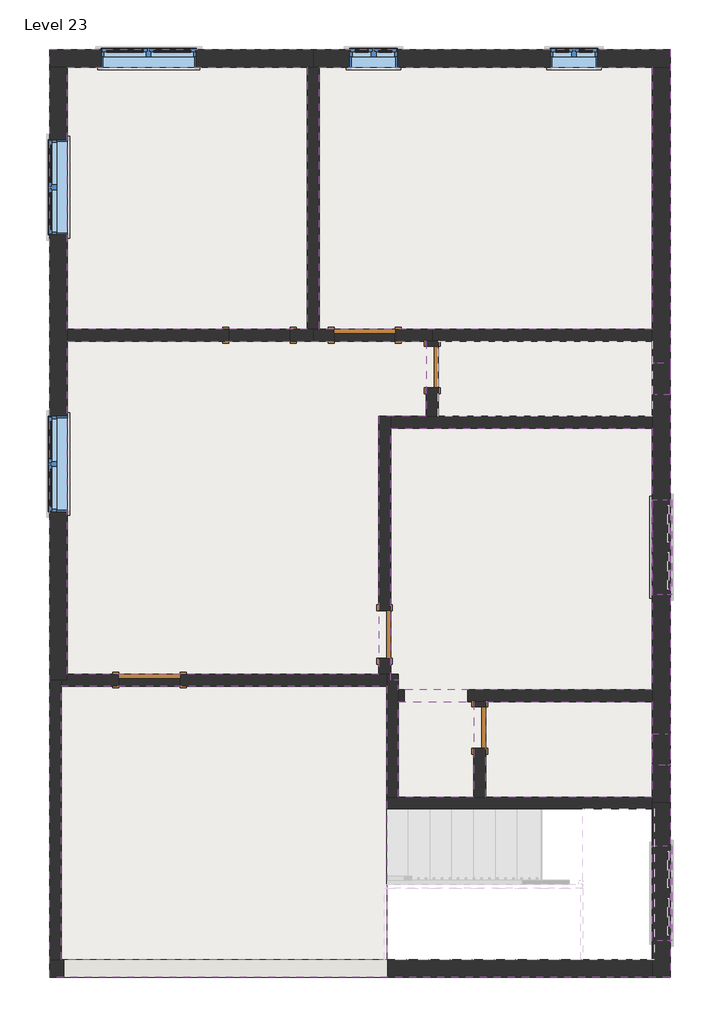
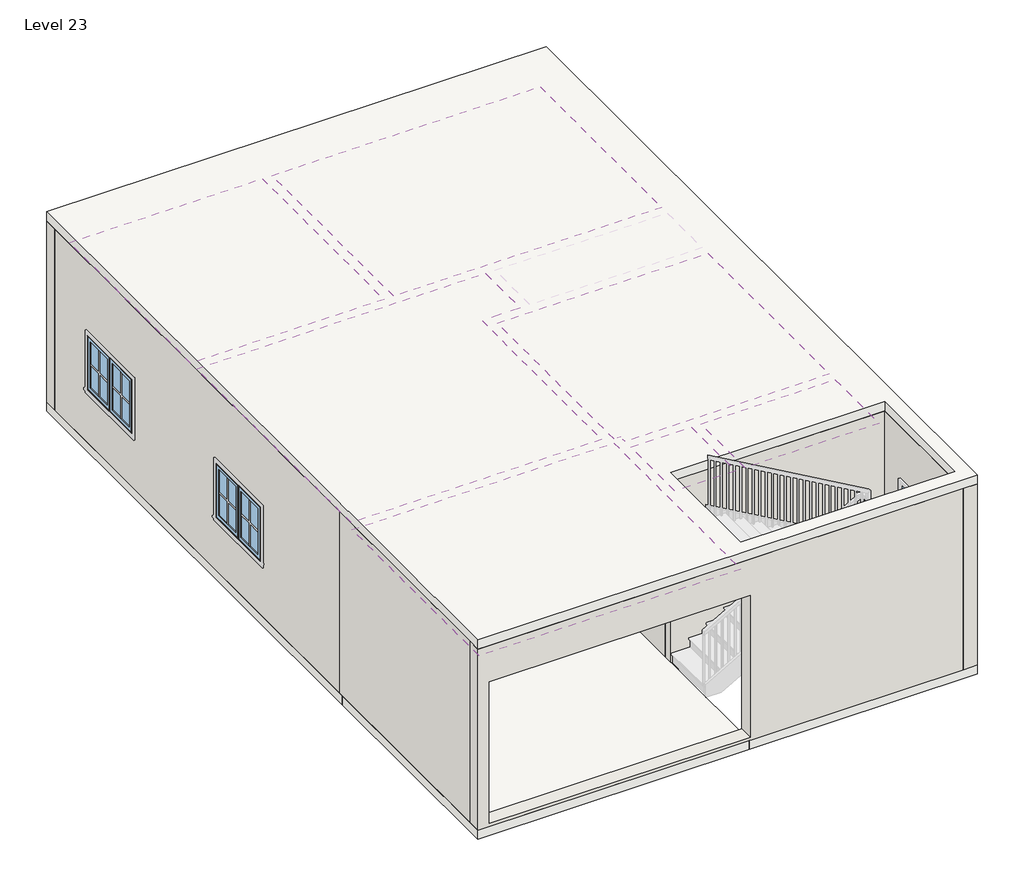
# One storey, part 1 of 2: 27 walls, 13 windows, 7 coverings, 6 doors, 3 slabs.
# Revit data of these elements (continued)
# Element 47 (IfcWindow, "Window-Casement-Double : 3'") (continued)
#   Materials on its faces: "Wood - Stained", "Glass", "Clad - White"
# Element 48 (IfcWindow, "Window-Casement-Double : 3'")
#   Mark = "103"
#   Window Inset = 0' - 0"
#   Interior Wall Closure = 0' - 2 1/4"
#   Frame Extension = 0' - 0 1/4"
#   Exterior Wall Closure = 0' - 1 1/4"
#   Interior Trim Visibility = yes
#   Exterior Trim Visibility = yes
#   Phase Created = New Construction
#   Materials on its faces: "Wood - Stained", "Glass", "Clad - White"
# Element 49 (IfcWindow, "Window-Casement-Double : 3'")
#   Mark = "104"
#   Window Inset = 0' - 0"
#   Interior Wall Closure = 0' - 2 1/4"
#   Frame Extension = 0' - 0 1/4"
#   Exterior Wall Closure = 0' - 1 1/4"
#   Interior Trim Visibility = yes
#   Exterior Trim Visibility = yes
#   Phase Created = New Construction
#   Materials on its faces: "Wood - Stained", "Glass", "Clad - White"
# Element 50 (IfcWindow, "Window-Casement-Double : 4'")
#   Mark = "92"
#   Window Inset = 0' - 0"
#   Interior Wall Closure = 0' - 2 1/4"
#   Frame Extension = 0' - 0 1/4"
#   Exterior Wall Closure = 0' - 1 1/4"
#   Interior Trim Visibility = yes
#   Exterior Trim Visibility = yes
#   Phase Created = New Construction
#   Materials on its faces: "Wood - Stained", "Glass", "Clad - White"
# Element 51 (IfcWindow, "Window-Casement-Double : 4'")
#   Mark = "93"
#   Window Inset = 0' - 0"
#   Interior Wall Closure = 0' - 2 1/4"
#   Frame Extension = 0' - 0 1/4"
#   Exterior Wall Closure = 0' - 1 1/4"
#   Interior Trim Visibility = yes
#   Exterior Trim Visibility = yes
#   Phase Created = New Construction
#   Materials on its faces: "Wood - Stained", "Glass", "Clad - White"
# Element 52 (IfcWindow, "Window-Casement-Double : 4'")
#   Mark = "94"
#   Window Inset = 0' - 0"
#   Interior Wall Closure = 0' - 2 1/4"
#   Frame Extension = 0' - 0 1/4"
#   Exterior Wall Closure = 0' - 1 1/4"
#   Interior Trim Visibility = yes
#   Exterior Trim Visibility = yes
#   Phase Created = New Construction
#   Materials on its faces: "Wood - Stained", "Glass", "Clad - White"
# Element 53 (IfcWindow, "Window-Casement-Double : 4'")
#   Mark = "95"
#   Window Inset = 0' - 0"
#   Interior Wall Closure = 0' - 2 1/4"
#   Frame Extension = 0' - 0 1/4"
#   Exterior Wall Closure = 0' - 1 1/4"
#   Interior Trim Visibility = yes
#   Exterior Trim Visibility = yes
#   Phase Created = New Construction
#   Materials on its faces: "Wood - Stained", "Glass", "Clad - White"
# Element 54 (IfcWindow, "Window-Casement-Double : 4'")
#   Mark = "96"
#   Window Inset = 0' - 0"
#   Interior Wall Closure = 0' - 2 1/4"
#   Frame Extension = 0' - 0 1/4"
#   Exterior Wall Closure = 0' - 1 1/4"
#   Interior Trim Visibility = yes
#   Exterior Trim Visibility = yes
#   Phase Created = New Construction
#   Materials on its faces: "Wood - Stained", "Glass", "Clad - White"
# Element 55 (IfcWindow, "Window-Casement-Double : 4'")
#   Mark = "101"
#   Window Inset = 0' - 0"
#   Interior Wall Closure = 0' - 2 1/4"
#   Frame Extension = 0' - 0 1/4"
#   Exterior Wall Closure = 0' - 1 1/4"
#   Interior Trim Visibility = yes
#   Exterior Trim Visibility = yes
#   Phase Created = New Construction
#   Materials on its faces: "Wood - Stained", "Glass", "Clad - White"
# Element 56 (IfcWindow, "Window-Casement-Double : 4'")
#   Mark = "102"
#   Window Inset = 0' - 0"
#   Interior Wall Closure = 0' - 2 1/4"
#   Frame Extension = 0' - 0 1/4"
#   Exterior Wall Closure = 0' - 1 1/4"
#   Interior Trim Visibility = yes
#   Exterior Trim Visibility = yes
#   Phase Created = New Construction
#   Materials on its faces: "Wood - Stained", "Glass", "Clad - White"
# Materials
#   "Default": colour RGB 127 127 127, transparency 0, Cost = 0
#   "Acoustic Ceiling Tile 24 x 48": class "Generic", colour RGB 229 229 229, transparency 0, Description = "Acoustic Ceiling Tile 24 x 48", Cost = 0
#   "Door - Panel": class "Wood", colour RGB 210 159 95, transparency 0, Cost = 0
#   "Door - Frame": colour RGB 118 70 51, transparency 0, Cost = 0
#   "Glass": class "Glass", colour RGB 0 128 192, transparency 0.75, Description = "Soda Lime Glass", Cost = 0
#   "Sash": class "Wood", colour RGB 224 178 126, transparency 0, Cost = 0
#   "Wood - Stained": class "Wood", colour RGB 224 178 126, transparency 0, Cost = 0
#   "Clad - White": class "Wood", colour RGB 242 242 238, transparency 0, Cost = 0
#   "Default Floor": colour RGB 128 128 128, transparency 0, Cost = 0
#   "TILE": class "Generic", colour RGB 120 120 120, transparency 0, Cost = 0
#   "Grass": class "Generic", colour RGB 104 137 66, transparency 0, Description = "Physical material.", Cost = 0
#   "Default Wall": colour RGB 128 128 128, transparency 0, Cost = 0
#   "WALL PAINT 4": class "Generic", colour RGB 120 120 120, transparency 0, Cost = 0
#   "MARBLE": class "Generic", colour RGB 120 120 120, transparency 0, Cost = 0
#   "WALL PAINT 5": class "Generic", colour RGB 120 120 120, transparency 0, Cost = 0
#   "WALL PAINT 2": class "Generic", colour RGB 120 120 120, transparency 0, Cost = 0
#   "WALL PAINT 3": class "Generic", colour RGB 120 120 120, transparency 0, Cost = 0
#   "WALL PAINT 1": class "Generic", colour RGB 120 120 120, transparency 0, Cost = 0
